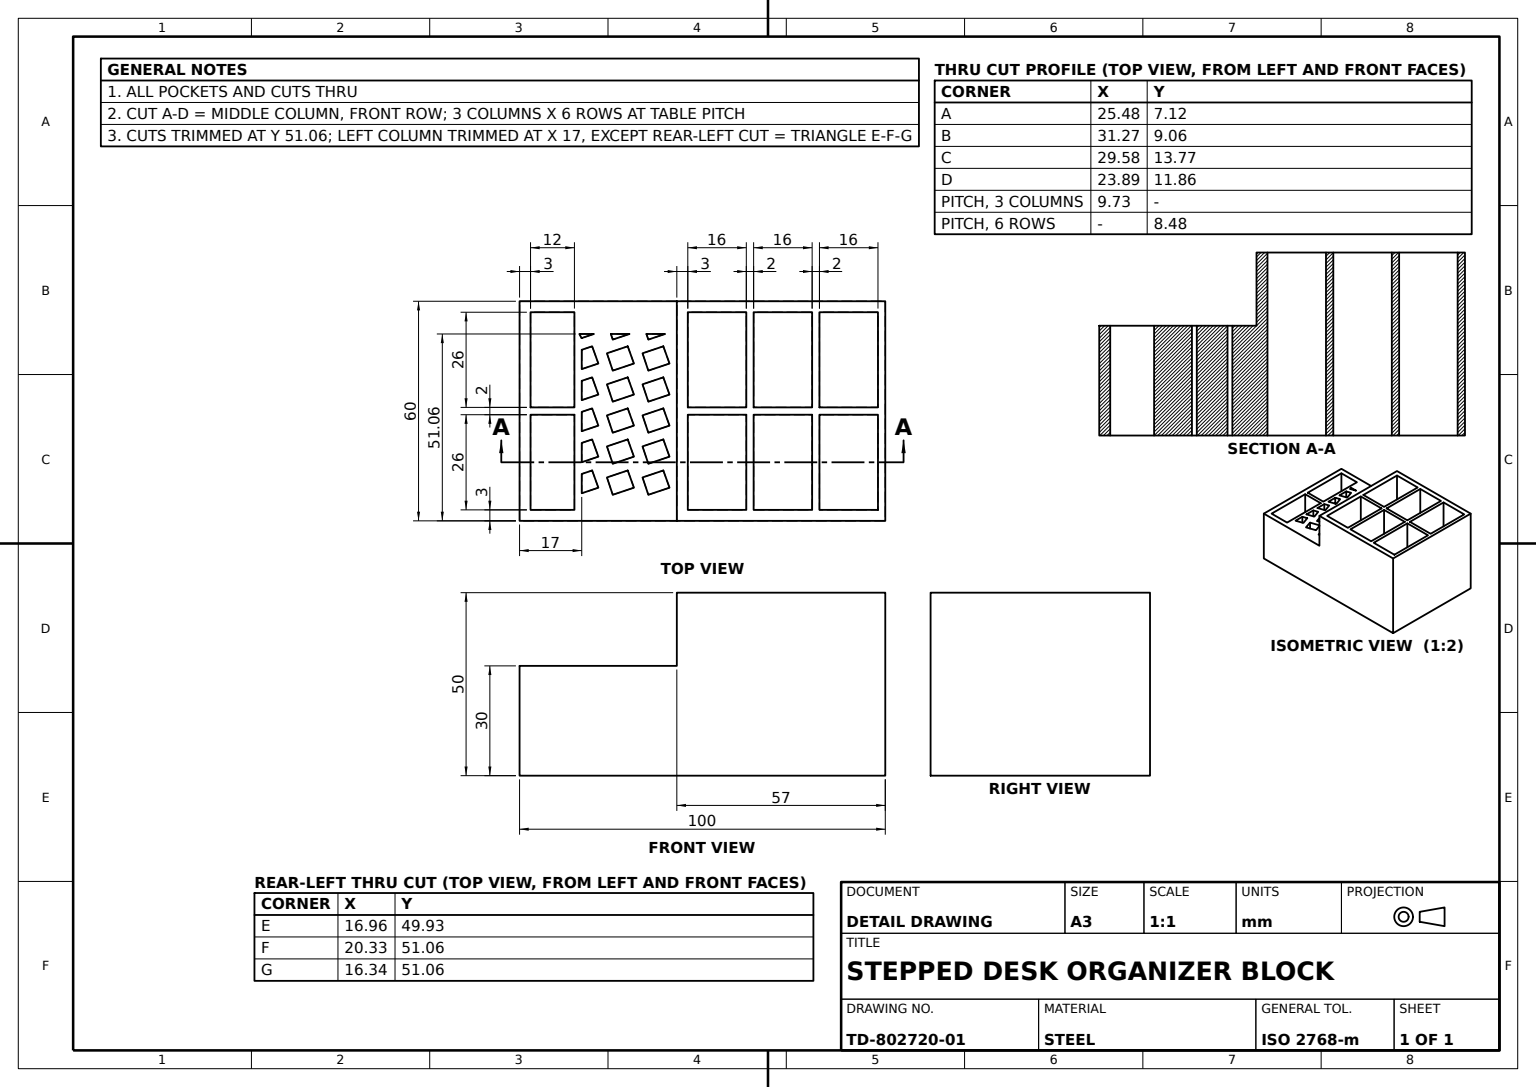
SolidWorks part; units mm, degrees
material "Plain Carbon Steel"
ref_plane "Front Plane" through (0, 0, 0) normal (0, 0, 1) x (1, 0, 0)
ref_plane "Top Plane" through (0, 0, 0) normal (0, 1, 0) x (1, 0, 0)
ref_plane "Right Plane" through (0, 0, 0) normal (1, 0, 0) x (0, 0, -1)
sketch "Stepped Block Profile" plane through (0, 0, 0) normal (0, 0, 1) x (1, 0, 0)
  line L0 (77.9974, 0) -> (-78.7879, 0) construction
  line L1 (0, 48.6825) -> (0, -50.7905) construction
  line L2 (-50, 5.5995) -> (50, 5.5995)
  line L3 (50, 5.5995) -> (50, 55.5995)
  line L4 (50, 55.5995) -> (-7, 55.5995)
  line L5 (-7, 55.5995) -> (-7, 35.5995)
  line L6 (-7, 35.5995) -> (-50, 35.5995)
  line L7 (-50, 35.5995) -> (-50, 5.5995)
  dimension "D1" = 100
  dimension "D2" = 57
  dimension "D3" = 30
  dimension "D4" = 50
  dimension "D5" = 35.5995
extrude "Stepped Block" add sketch "Stepped Block Profile" along normal mid plane 60
sketch "Lower Step Pockets Sketch" plane through (0, 55.5995, 0) normal (0, 1, 0) x (1, 0, 0)
  line L0 (-7, -30) -> (-7, 30) construction
  line L1 (-4, -1) -> (12, -1)
  line L2 (-4, -1) -> (-4, -27)
  line L3 (-4, -27) -> (12, -27)
  line L4 (12, -1) -> (12, -27)
  line L5 (-4, -1) -> (12, -27) construction
  line L6 (-4, -27) -> (12, -1) construction
  line L7 (50, -30) -> (-7, -30) construction
  line L8 (14, -1) -> (14, -27)
  line L9 (14, -1) -> (30, -1)
  line L10 (14, -27) -> (30, -27)
  line L11 (30, -1) -> (30, -27)
  line L12 (32, -1) -> (32, -27)
  line L13 (32, -1) -> (48, -1)
  line L14 (48, -1) -> (48, -27)
  line L15 (32, -27) -> (48, -27)
  line L16 (-13.3552, 0) -> (66.3174, 0) construction
  line L17 (32, 1) -> (48, 1)
  line L18 (48, 1) -> (48, 27)
  line L19 (32, 27) -> (48, 27)
  line L20 (32, 1) -> (32, 27)
  line L21 (14, 1) -> (30, 1)
  line L22 (30, 1) -> (30, 27)
  line L23 (14, 27) -> (30, 27)
  line L24 (14, 1) -> (14, 27)
  line L25 (-4, 27) -> (12, 27)
  line L26 (12, 1) -> (12, 27)
  line L27 (-4, 1) -> (12, 1)
  line L28 (-4, 1) -> (-4, 27)
  point P0 (4, -14)
  dimension "D1" = 16
  dimension "D2" = 3
  dimension "D3" = 26
  dimension "D4" = 3
  dimension "D5" = 2
  dimension "D6" = 2
  dimension "D7" = 26
  dimension "D8" = 26
extrude "Lower Step Pockets" cut sketch "Lower Step Pockets Sketch" against normal through all
sketch "Upper Step Pockets Sketch" plane through (0, 35.5995, 0) normal (0, 1, 0) x (1, 0, 0)
  line L0 (-50, -30) -> (-50, 30) construction
  line L1 (-47, -27) -> (-35, -27)
  line L2 (-47, -27) -> (-47, -1)
  line L3 (-47, -1) -> (-35, -1)
  line L4 (-35, -27) -> (-35, -1)
  line L5 (-47, -27) -> (-35, -1) construction
  line L6 (-47, -1) -> (-35, -27) construction
  line L7 (-7, -30) -> (-50, -30) construction
  line L8 (0, 0) -> (-66.9715, 0) construction
  line L9 (-47, 1) -> (-35, 1)
  line L10 (-35, 27) -> (-35, 1)
  line L11 (-47, 27) -> (-35, 27)
  line L12 (-47, 27) -> (-47, 1)
  point P0 (-41, -14)
  dimension "D1" = 3
  dimension "D2" = 3
  dimension "D3" = 26
  dimension "D4" = 12
extrude "Upper Step Pockets" cut sketch "Upper Step Pockets Sketch" against normal through all
sketch "Triangular Cuts Sketch" plane through (0, 35.5995, 0) normal (0, 1, 0) x (1, 0, 0)
  line L0 (-33.6634, 21.0601) -> (-29.667, 21.0601)
  line L1 (-33, 16.7344) -> (-33, 11.4624)
  line L4 (-35, -27) -> (-35, -1) construction
  line L5 (-47, -1) -> (-47, -27) construction
  line L6 (-35, -1) -> (-47, -1) construction
  line L8 (-18.7289, -20.9393) -> (-24.5215, -22.8801)
  line L9 (-9, -20.9393) -> (-14.7926, -22.8801)
  line L10 (-24.5215, -22.8801) -> (-26.1096, -18.1403)
  line L11 (-14.7926, -22.8801) -> (-16.3807, -18.1403)
  line L12 (-16.3807, -18.1403) -> (-10.6915, -16.2341)
  line L13 (-10.6915, -16.2341) -> (-9, -20.9393)
  line L14 (-26.1096, -18.1403) -> (-20.4205, -16.2341)
  line L15 (-20.4205, -16.2341) -> (-18.7289, -20.9393)
  line L17 (-28.4579, -20.9393) -> (-33, -22.4611)
  line L19 (-33, -17.1892) -> (-30.1494, -16.2341)
  line L20 (-30.1494, -16.2341) -> (-28.4579, -20.9393)
  line L22 (-18.7289, -12.4584) -> (-24.5215, -14.3992)
  line L23 (-24.5215, -14.3992) -> (-26.1096, -9.6594)
  line L24 (-26.1096, -9.6594) -> (-20.4205, -7.7532)
  line L25 (-20.4205, -7.7532) -> (-18.7289, -12.4584)
  line L26 (-33, 8.2535) -> (-33, 2.9815)
  line L27 (-28.4579, -12.4584) -> (-33, -13.9802)
  line L29 (-33, -8.7083) -> (-30.1494, -7.7532)
  line L30 (-30.1494, -7.7532) -> (-28.4579, -12.4584)
  line L32 (-18.7289, -3.9775) -> (-24.5215, -5.9183)
  line L33 (-24.5215, -5.9183) -> (-26.1096, -1.1785)
  line L34 (-26.1096, -1.1785) -> (-20.4205, 0.7277)
  line L35 (-20.4205, 0.7277) -> (-18.7289, -3.9775)
  line L37 (-28.4579, -3.9775) -> (-33, -5.4994)
  line L39 (-33, -0.2274) -> (-30.1494, 0.7277)
  line L40 (-30.1494, 0.7277) -> (-28.4579, -3.9775)
  line L42 (-18.7289, 4.5034) -> (-24.5215, 2.5626)
  line L43 (-24.5215, 2.5626) -> (-26.1096, 7.3024)
  line L44 (-26.1096, 7.3024) -> (-20.4205, 9.2086)
  line L45 (-20.4205, 9.2086) -> (-18.7289, 4.5034)
  line L47 (-28.4579, 4.5034) -> (-33, 2.9815)
  line L49 (-33, 8.2535) -> (-30.1494, 9.2086)
  line L50 (-30.1494, 9.2086) -> (-28.4579, 4.5034)
  line L52 (-18.7289, 12.9843) -> (-24.5215, 11.0434)
  line L53 (-24.5215, 11.0434) -> (-26.1096, 15.7833)
  line L54 (-26.1096, 15.7833) -> (-20.4205, 17.6895)
  line L55 (-20.4205, 17.6895) -> (-18.7289, 12.9843)
  line L57 (-28.4579, 12.9843) -> (-33, 11.4624)
  line L59 (-33, 16.7344) -> (-30.1494, 17.6895)
  line L60 (-30.1494, 17.6895) -> (-28.4579, 12.9843)
  line L62 (-19.938, 21.0601) -> (-24.5215, 19.5243)
  line L63 (-24.5215, 19.5243) -> (-25.0361, 21.0601)
  line L67 (-29.667, 21.0601) -> (-33.0417, 19.9294)
  line L72 (-9, -12.4584) -> (-14.7926, -14.3992)
  line L73 (-14.7926, -14.3992) -> (-16.3807, -9.6594)
  line L74 (-16.3807, -9.6594) -> (-10.6915, -7.7532)
  line L75 (-10.6915, -7.7532) -> (-9, -12.4584)
  line L77 (-9, -3.9775) -> (-14.7926, -5.9183)
  line L78 (-14.7926, -5.9183) -> (-16.3807, -1.1785)
  line L79 (-16.3807, -1.1785) -> (-10.6915, 0.7277)
  line L80 (-10.6915, 0.7277) -> (-9, -3.9775)
  line L81 (-33, -0.2274) -> (-33, -5.4994)
  line L82 (-9, 4.5034) -> (-14.7926, 2.5626)
  line L83 (-14.7926, 2.5626) -> (-16.3807, 7.3024)
  line L84 (-16.3807, 7.3024) -> (-10.6915, 9.2086)
  line L85 (-10.6915, 9.2086) -> (-9, 4.5034)
  line L86 (-33, -8.7083) -> (-33, -13.9802)
  line L87 (-9, 12.9843) -> (-14.7926, 11.0434)
  line L88 (-14.7926, 11.0434) -> (-16.3807, 15.7833)
  line L89 (-16.3807, 15.7833) -> (-10.6915, 17.6895)
  line L90 (-10.6915, 17.6895) -> (-9, 12.9843)
  line L91 (-33, -17.1892) -> (-33, -22.4611)
  line L92 (-10.2091, 21.0601) -> (-14.7926, 19.5243)
  line L93 (-14.7926, 19.5243) -> (-15.3072, 21.0601)
  line L96 (-25.0361, 21.0601) -> (-19.938, 21.0601)
  line L97 (-33, 54.9836) -> (-29, 54.9836) [skipped]
  line L98 (-43, 54.9836) -> (-33, 54.9836) [skipped]
  line L99 (-43.3077, 29.541) -> (-18.972, 29.541) [skipped]
  line L100 (-62.2387, 29.541) -> (-37.903, 29.541) [skipped]
  line L101 (-43.3077, 38.0219) -> (-18.972, 38.0219) [skipped]
  line L102 (-62.2387, 38.0219) -> (-37.903, 38.0219) [skipped]
  line L103 (-43.3077, 46.5027) -> (-18.972, 46.5027) [skipped]
  line L104 (-62.2387, 46.5027) -> (-37.903, 46.5027) [skipped]
  line L105 (-66.319, 54.9836) -> (-46.319, 54.9836) [skipped]
  line L106 (-34.1509, 63.4645) -> (-9.8152, 63.4645) [skipped]
  line L107 (-53.0639, 63.4645) -> (-28.7282, 63.4645) [skipped]
  line L108 (-33.3357, 29.541) -> (-9, 29.541) [skipped]
  line L109 (-33.3357, 38.0219) -> (-9, 38.0219) [skipped]
  line L110 (-33.3357, 46.5027) -> (-9, 46.5027) [skipped]
  line L111 (-24.1789, 63.4645) -> (0.1568, 63.4645) [skipped]
  line L112 (-35.8386, 24.2642) -> (-30.1494, 26.1703) [skipped]
  line L113 (-30.1494, 26.1703) -> (-28.4579, 21.4652) [skipped]
  line L114 (-43, 21.0601) -> (-36.738, 21.0601) [skipped]
  line L115 (-36.7309, 26.9274) -> (-36.91, 27.462) [skipped]
  line L116 (-26.1096, 24.2642) -> (-20.4205, 26.1703) [skipped]
  line L117 (-20.4205, 26.1703) -> (-18.7289, 21.4652) [skipped]
  line L118 (-16.3807, 24.2642) -> (-10.6915, 26.1703) [skipped]
  line L119 (-10.6915, 26.1703) -> (-9, 21.4652) [skipped]
  line L120 (-34.2505, 11.0434) -> (-35.8386, 15.7833) [skipped]
  line L121 (-34.2505, 2.5626) -> (-35.8386, 7.3024) [skipped]
  line L122 (-34.2505, -5.9183) -> (-35.8386, -1.1785) [skipped]
  line L123 (-34.2505, -14.3992) -> (-35.8386, -9.6594) [skipped]
  line L124 (-34.2505, -22.8801) -> (-35.8386, -18.1403) [skipped]
  line L125 (-15.3072, 21.0601) -> (-10.2091, 21.0601)
  line L126 (-33.0417, 19.9294) -> (-33.6634, 21.0601)
  line L128 (-42.3374, 21.0601) -> (-40.0242, 21.0601) [skipped]
  dimension "D1" = 2
  dimension "D2" = 0.681
  dimension "D5" = 3
  dimension "D6" = 6
  dimension "D7" = 4.6626
  dimension "D8" = 5
  dimension "D9" = 6
  dimension "D10" = 90
  dimension "D11" = 6.9758
  dimension "D12" = 3.6923
  dimension "D13" = 10.09
  dimension "D14" = 10.262
  dimension "D15" = 10.2691
  dimension "D16" = 4
  dimension "D17" = 9.097
  dimension "D18" = 12.8491
  dimension "D19" = 13.3366
  dimension "D20" = 11.1614
  dimension "D21" = 13.9583
  dimension "D22" = 12.7495
  dimension "D23" = 13.6643
  dimension "D24" = 18
  dimension "D25" = 18.2718
  dimension "D26" = 16.8506
  dimension "D27" = 17.333
  dimension "D28" = 18.5421
  dimension "D29" = 20.8904
  dimension "D30" = 22.8211
  dimension "D31" = 28.028
  dimension "D32" = 47.1568
  dimension "D33" = 15.2387
  dimension "D34" = 0.7726
  dimension "D35" = 3.5626
  dimension "D40" = 37.1848
  dimension "D43" = 6.0639
  dimension "D45" = 19.319
extrude "Triangular Cuts" cut sketch "Triangular Cuts Sketch" against normal up to surface (30 mm away) up to face at (-41, 5.5995, 14)
